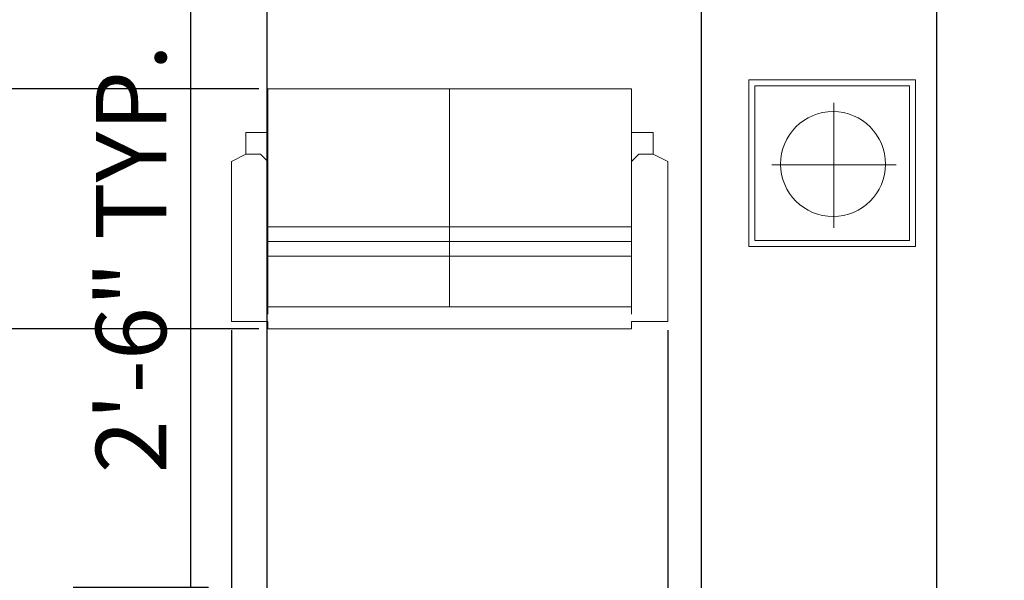
# Model space of a CAD drawing. Units: inches. Extents: x 2923 to 3500, y 1684 to 2381.
# Tile 4 of 12: x 3176 to 3246, y 1848 to 1888. Entities that reach past the tile are written whole.
import ezdxf

# ---------------------------------------------------------------- set-up
doc = ezdxf.new("R2010")
doc.units = ezdxf.units.IN
doc.layers.add('A-ANNO-DIMS', color=2, linetype='Continuous', lineweight=18)
doc.layers.add('Furniture', color=7, linetype='Continuous', lineweight=15)
doc.styles.get("Standard").update_dxf_attribs({"font": 'txt', "height": 5})
doc.dimstyles.new('ISO-25', dxfattribs={"dimtxt": 5, "dimasz": 2.5, "dimexe": 1.25, "dimexo": 0.625, "dimtad": 1, "dimlunit": 3, "dimtxsty": 'Standard', "dimcen": 2.5, "dimadec": 0, "dimazin": 0, "dimtfac": 1, "dimtmove": 0, "dimatfit": 3, "dimfxl": 1, "dimarcsym": 0})

# ---------------------------------------------------------------- blocks, each defined once
blk = doc.blocks.new('TABLE-END')
for p, q in [((0, 0), (0, 11.85)), ((0, 11.85), (11.85, 11.85)), ((0.431, 0.431), (0.431, 11.419)), ((0.431, 11.419), (11.419, 11.419)), ((11.419, 11.419), (11.419, 0.431)), ((11.85, 11.85), (11.85, 0)), ((6.027, 10.204), (6.027, 1.328)), ((10.468, 5.813), (1.634, 5.813)), ((11.85, 0), (0, 0)), ((11.419, 0.431), (0.431, 0.431))]:
    blk.add_line(p, q)
blk.add_circle((5.98, 5.861), 3.73)
blk = doc.blocks.new('*D30')
at = {"layer": 'A-ANNO-DIMS', "color": 0, "lineweight": -2, "transparency": 16777216}
for p, q in [((3188.23, 1847.406), (3188.23, 1891.632)), ((3179.855, 1847.406), (3189.48, 1847.406)), ((3188.23, 1819.906), (3188.23, 1844.906)), ((3179.855, 1817.406), (3189.48, 1817.406))]:
    blk.add_line(p, q, dxfattribs=at)
at = {"layer": 'A-ANNO-DIMS', "color": 0, "transparency": 16777216}
for points in [[(3187.813, 1844.906), (3188.646, 1844.906), (3188.23, 1847.406)], [(3187.813, 1819.906), (3188.646, 1819.906), (3188.23, 1817.406)]]:
    blk.add_solid(points, dxfattribs=at)
at = {"layer": 'Defpoints', "color": 0, "transparency": 16777216}
for p in [(3179.23, 1847.406), (3188.23, 1847.406), (3179.23, 1817.406)]:
    blk.add_point(p, dxfattribs=at)
at = {"layer": 'A-ANNO-DIMS', "color": 0, "transparency": 16777216, "insert": (3184.629, 1870.769), "char_height": 5, "attachment_point": 5, "rotation": 90}
blk.add_mtext('2\'-6" TYP.', dxfattribs=at)
blk = doc.blocks.new('*D54')
at = {"layer": 'A-ANNO-DIMS', "color": 0, "lineweight": -2, "transparency": 16777216}
for p, q in [((3166.316, 2236.755), (3166.316, 1685.656)), ((3193.644, 2236.755), (3193.644, 1685.656)), ((3168.816, 1686.906), (3191.144, 1686.906)), ((3193.644, 1686.906), (3235.489, 1686.906))]:
    blk.add_line(p, q, dxfattribs=at)
at = {"layer": 'A-ANNO-DIMS', "color": 0, "transparency": 16777216}
for points in [[(3168.816, 1687.323), (3168.816, 1686.49), (3166.316, 1686.906)], [(3191.144, 1687.323), (3191.144, 1686.49), (3193.644, 1686.906)]]:
    blk.add_solid(points, dxfattribs=at)
at = {"layer": 'Defpoints', "color": 0, "transparency": 16777216}
for p in [(3166.316, 2237.38), (3193.644, 2237.38), (3193.644, 1686.906)]:
    blk.add_point(p, dxfattribs=at)
at = {"layer": 'A-ANNO-DIMS', "color": 0, "transparency": 16777216, "insert": (3215.817, 1691.341), "char_height": 5, "attachment_point": 5}
blk.add_mtext('2\'-3 1/2"', dxfattribs=at)
blk = doc.blocks.new('*D61')
at = {"layer": 'A-ANNO-DIMS', "color": 0, "lineweight": -2, "transparency": 16777216}
for p, q in [((3224.497, 1890.49), (3224.497, 1685.656)), ((3241.226, 1890.49), (3241.226, 1685.656)), ((3226.997, 1686.906), (3238.726, 1686.906)), ((3241.226, 1686.906), (3282.119, 1686.906))]:
    blk.add_line(p, q, dxfattribs=at)
at = {"layer": 'A-ANNO-DIMS', "color": 0, "transparency": 16777216}
for points in [[(3226.997, 1687.323), (3226.997, 1686.49), (3224.497, 1686.906)], [(3238.726, 1687.323), (3238.726, 1686.49), (3241.226, 1686.906)]]:
    blk.add_solid(points, dxfattribs=at)
at = {"layer": 'Defpoints', "color": 0, "transparency": 16777216}
for p in [(3224.497, 1891.115), (3241.226, 1891.115), (3241.226, 1686.906)]:
    blk.add_point(p, dxfattribs=at)
at = {"layer": 'A-ANNO-DIMS', "color": 0, "transparency": 16777216, "insert": (3262.923, 1691.341), "char_height": 5, "attachment_point": 5}
blk.add_mtext('1\'-4 1/2"', dxfattribs=at)
blk = doc.blocks.new('*D64')
at = {"layer": 'A-ANNO-DIMS', "color": 0, "lineweight": -2, "transparency": 16777216}
for p, q in [((3191.114, 1865.68), (3191.114, 1685.656)), ((3222.138, 1865.68), (3222.138, 1685.656)), ((3193.614, 1686.906), (3219.638, 1686.906))]:
    blk.add_line(p, q, dxfattribs=at)
at = {"layer": 'A-ANNO-DIMS', "color": 0, "transparency": 16777216}
for points in [[(3193.614, 1687.323), (3193.614, 1686.49), (3191.114, 1686.906)], [(3219.638, 1687.323), (3219.638, 1686.49), (3222.138, 1686.906)]]:
    blk.add_solid(points, dxfattribs=at)
at = {"layer": 'Defpoints', "color": 0, "transparency": 16777216}
for p in [(3191.114, 1866.305), (3222.138, 1866.305), (3222.138, 1686.906)]:
    blk.add_point(p, dxfattribs=at)
at = {"layer": 'A-ANNO-DIMS', "color": 0, "transparency": 16777216, "insert": (3206.626, 1690.507), "char_height": 5, "attachment_point": 5}
blk.add_mtext('2\'-7"', dxfattribs=at)
blk = doc.blocks.new('*D65')
at = {"layer": 'A-ANNO-DIMS', "color": 0, "lineweight": -2, "transparency": 16777216}
for p, q in [((2934.73, 1882.852), (2934.73, 1905.411)), ((3193.074, 1882.852), (2933.48, 1882.852)), ((2934.73, 1868.288), (2934.73, 1880.352)), ((3193.074, 1865.788), (2933.48, 1865.788))]:
    blk.add_line(p, q, dxfattribs=at)
at = {"layer": 'A-ANNO-DIMS', "color": 0, "transparency": 16777216}
for points in [[(2934.313, 1880.352), (2935.146, 1880.352), (2934.73, 1882.852)], [(2934.313, 1868.288), (2935.146, 1868.288), (2934.73, 1865.788)]]:
    blk.add_solid(points, dxfattribs=at)
at = {"layer": 'Defpoints', "color": 0, "transparency": 16777216}
for p in [(2934.73, 1882.852), (3193.699, 1882.852), (3193.699, 1865.788)]:
    blk.add_point(p, dxfattribs=at)
at = {"layer": 'A-ANNO-DIMS', "color": 0, "transparency": 16777216, "insert": (2931.129, 1895.382), "char_height": 5, "attachment_point": 5, "rotation": 90}
blk.add_mtext('1\'-5"', dxfattribs=at)

msp = doc.modelspace()

# ---------------------------------------------------------------- linework, layer by layer
at = {"layer": 'Furniture'}
for p, q in [((3193.699, 1882.852), (3219.553, 1882.852)), ((3193.699, 1879.749), (3193.699, 1882.852)), ((3206.626, 1882.852), (3206.626, 1867.34)), ((3219.553, 1882.852), (3219.553, 1879.749)), ((3192.148, 1878.198), (3192.148, 1879.749)), ((3192.148, 1879.749), (3193.699, 1879.749)), ((3193.699, 1879.749), (3193.699, 1877.681)), ((3219.553, 1879.749), (3219.553, 1877.681)), ((3219.553, 1879.749), (3221.104, 1879.749)), ((3221.104, 1879.749), (3221.104, 1878.198)), ((3191.114, 1877.681), (3192.148, 1878.198)), ((3192.148, 1878.198), (3193.182, 1878.198)), ((3193.182, 1878.198), (3193.699, 1877.681)), ((3220.07, 1878.198), (3219.553, 1877.681)), ((3221.104, 1878.198), (3220.07, 1878.198)), ((3221.104, 1878.198), (3222.138, 1877.681)), ((3191.114, 1866.305), (3191.114, 1877.681)), ((3193.699, 1877.681), (3193.699, 1866.822)), ((3219.553, 1877.681), (3219.553, 1866.822)), ((3222.138, 1877.681), (3222.138, 1866.305)), ((3193.699, 1873.027), (3219.553, 1873.027)), ((3193.699, 1871.993), (3219.553, 1871.993)), ((3193.699, 1870.959), (3219.553, 1870.959)), ((3219.553, 1867.34), (3193.699, 1867.34)), ((3193.699, 1866.305), (3191.114, 1866.305)), ((3193.699, 1865.788), (3193.699, 1866.305)), ((3222.138, 1866.305), (3219.553, 1866.305)), ((3219.553, 1866.305), (3219.553, 1865.788)), ((3219.553, 1865.788), (3193.699, 1865.788))]:
    msp.add_line(p, q, dxfattribs=at)

# ---------------------------------------------------------------- block references
msp.add_blockref('TABLE-END', (3227.902, 1871.638), dxfattribs=at)

# ---------------------------------------------------------------- dimensions: what is measured, and where the dimension line sits
at = {"layer": 'A-ANNO-DIMS'}
for base, p1, p2, picture, middle in [((3193.644, 1686.906), (3166.316, 2237.38), (3193.644, 2237.38), '*D54', (3215.817, 1691.341)), ((3241.226, 1686.906), (3224.497, 1891.115), (3241.226, 1891.115), '*D61', (3262.923, 1691.341)), ((3222.138, 1686.906), (3191.114, 1866.305), (3222.138, 1866.305), '*D64', (3206.626, 1690.507))]:
    dim = msp.add_linear_dim(base=base, p1=p1, p2=p2, dimstyle='ISO-25', override={"dimdec": 1, "dimlfac": 1, "dimrnd": 0, "dimzin": 1, "dimdsep": 46, "dimlunit": 4, "dimfrac": 2}, dxfattribs=at)
    dim.commit()
    dim.dimension.update_dxf_attribs({"geometry": picture, "text_midpoint": middle})
dim = msp.add_linear_dim(base=(2934.73, 1882.852), p1=(3193.699, 1865.788), p2=(3193.699, 1882.852), angle=90, dimstyle='ISO-25', override={"dimdec": 1, "dimlfac": 1, "dimrnd": 0, "dimzin": 1, "dimdsep": 46, "dimlunit": 4, "dimfrac": 2}, dxfattribs=at)
dim.commit()
dim.dimension.update_dxf_attribs({"geometry": '*D65', "text_midpoint": (2931.129, 1895.382)})
dim = msp.add_linear_dim(base=(3188.23, 1847.406), p1=(3179.23, 1817.406), p2=(3179.23, 1847.406), angle=90, text='<> TYP.', dimstyle='ISO-25', override={"dimdec": 1, "dimlfac": 1, "dimrnd": 0, "dimzin": 1, "dimdsep": 46, "dimlunit": 4, "dimfrac": 2}, dxfattribs=at)
dim.commit()
dim.dimension.update_dxf_attribs({"geometry": '*D30', "text_midpoint": (3184.629, 1870.769)})

doc.saveas('drawing.dxf')
